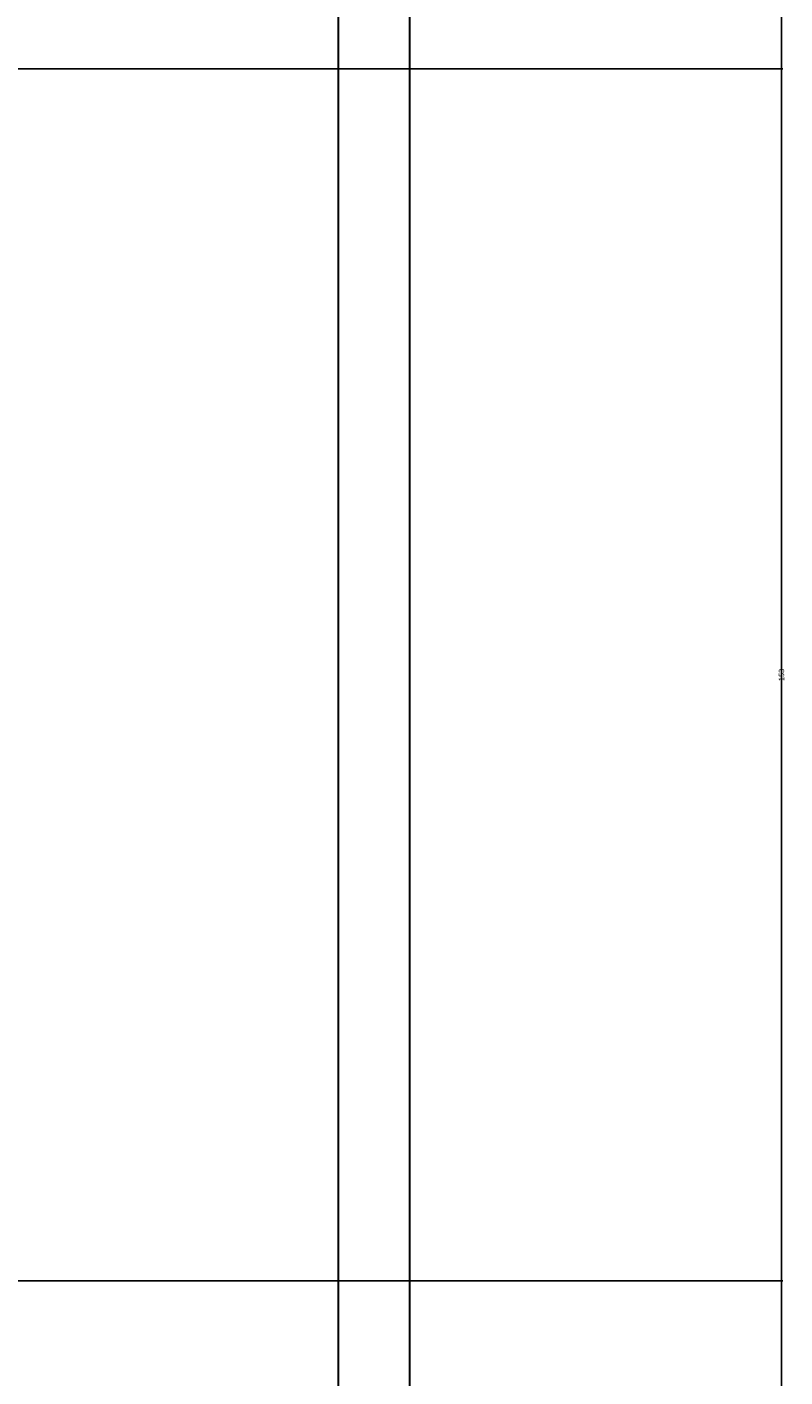
# Model space of a CAD drawing. Units: inches. Extents: x 867 to 1667, y -234 to 788.
# Tile 41 of 42: x 1572 to 1667, y 401 to 572. Entities that reach past the tile are written whole.
import ezdxf

# ---------------------------------------------------------------- set-up
doc = ezdxf.new("R2010")
doc.units = ezdxf.units.IN
doc.header["$MEASUREMENT"] = 0
doc.layers.add('A-ANNO-DIMS', color=2, linetype='Continuous', lineweight=18)
doc.layers.add('A-WALL-SITE', color=8, linetype='Continuous', lineweight=30)
doc.styles.get("Standard").update_dxf_attribs({"font": 'arial.ttf'})
doc.dimstyles.get("Standard").update_dxf_attribs({"dimtxt": 0.6875, "dimasz": 0.18, "dimexe": 0.18, "dimexo": 0.0625, "dimgap": 0.09, "dimtad": 0, "dimdec": 4, "dimzin": 0, "dimdsep": 46, "dimlunit": 4, "dimtxsty": 'Standard', "dimcen": 0.09, "dimadec": 0, "dimazin": 0, "dimtfac": 1, "dimtdec": 4, "dimtofl": 0, "dimtmove": 0, "dimatfit": 3, "dimfxl": 1, "dimtolj": 1, "dimtzin": 0, "dimarcsym": 0})

# ---------------------------------------------------------------- blocks, each defined once
blk = doc.blocks.new('*D18')
at = {"layer": 'A-ANNO-DIMS', "color": 0, "lineweight": -2, "transparency": 16777216}
for p, q in [((1619.95, 740.62), (1667.02, 740.62)), ((1666.84, 740.44), (1666.84, 277.95)), ((1666.84, -186.23), (1666.84, 276.25)), ((1619.95, -186.41), (1667.02, -186.41))]:
    blk.add_line(p, q, dxfattribs=at)
at = {"layer": 'A-ANNO-DIMS', "color": 0, "transparency": 16777216}
for points in [[(1666.81, 740.44), (1666.87, 740.44), (1666.84, 740.62)], [(1666.81, -186.23), (1666.87, -186.23), (1666.84, -186.41)]]:
    blk.add_solid(points, dxfattribs=at)
at = {"layer": 'Defpoints', "color": 0, "transparency": 16777216}
for p in [(1619.89, 740.62), (1666.84, 740.62), (1619.89, -186.41)]:
    blk.add_point(p, dxfattribs=at)
at = {"layer": 'A-ANNO-DIMS', "color": 0, "transparency": 16777216, "insert": (1666.84, 277.1), "char_height": 0.688, "attachment_point": 5, "rotation": 90}
blk.add_mtext('\\A1;927', dxfattribs=at)
blk = doc.blocks.new('*D34')
at = {"layer": 'A-ANNO-DIMS', "color": 0, "lineweight": -2, "transparency": 16777216}
for p, q in [((1538.95, 566.62), (1667.02, 566.62)), ((1666.84, 566.44), (1666.84, 490.93)), ((1666.84, 413.8), (1666.84, 489.3)), ((1538.95, 413.62), (1667.02, 413.62))]:
    blk.add_line(p, q, dxfattribs=at)
at = {"layer": 'A-ANNO-DIMS', "color": 0, "transparency": 16777216}
for points in [[(1666.81, 566.44), (1666.87, 566.44), (1666.84, 566.62)], [(1666.81, 413.8), (1666.87, 413.8), (1666.84, 413.62)]]:
    blk.add_solid(points, dxfattribs=at)
at = {"layer": 'Defpoints', "color": 0, "transparency": 16777216}
for p in [(1538.89, 566.62), (1666.84, 566.62), (1538.89, 413.62)]:
    blk.add_point(p, dxfattribs=at)
at = {"layer": 'A-ANNO-DIMS', "color": 0, "transparency": 16777216, "insert": (1666.84, 490.12), "char_height": 0.688, "attachment_point": 5, "rotation": 90}
blk.add_mtext('\\A1;153', dxfattribs=at)

msp = doc.modelspace()

# ---------------------------------------------------------------- linework, layer by layer
at = {"layer": 'A-WALL-SITE'}
for p, q in [((1610.8866, 740.617), (1610.8866, -186.4081)), ((1619.8866, 740.617), (1619.8866, -186.4081))]:
    msp.add_line(p, q, dxfattribs=at)

# ---------------------------------------------------------------- dimensions: what is measured, and where the dimension line sits
at = {"layer": 'A-ANNO-DIMS'}
for base, p1, p2, picture, middle in [((1666.8366, 740.617), (1619.8866, -186.4081), (1619.8866, 740.617), '*D18', (1666.8366, 277.1045)), ((1666.8366, 566.617), (1538.8866, 413.617), (1538.8866, 566.617), '*D34', (1666.8366, 490.117))]:
    dim = msp.add_linear_dim(base=base, p1=p1, p2=p2, angle=90, dimstyle='Standard', override={"dimdec": 0, "dimlfac": 1, "dimrnd": 0, "dimzin": 0, "dimdsep": 46, "dimlunit": 2}, dxfattribs=at)
    dim.commit()
    dim.dimension.update_dxf_attribs({"geometry": picture, "text_midpoint": middle})

doc.saveas('drawing.dxf')
